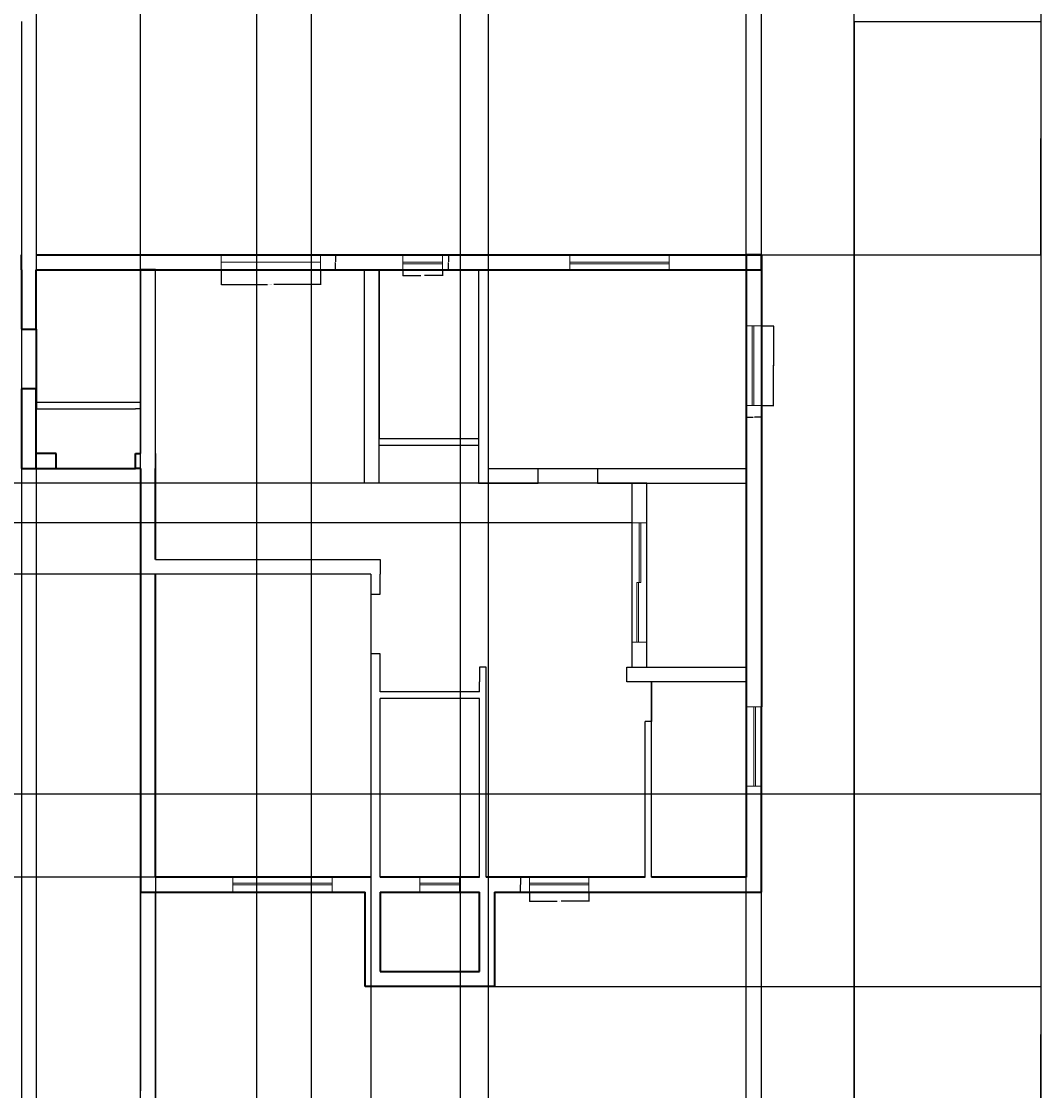
# Model space of a CAD drawing. Units: inches. Extents: x 2029 to 8798, y 1998 to 6373.
# Tile 9 of 11: x 3888 to 4504, y 5168 to 5814. Entities that reach past the tile are written whole.
import ezdxf

# ---------------------------------------------------------------- set-up
doc = ezdxf.new("R2010")
doc.units = ezdxf.units.IN
for name, color, linetype, lineweight in [('A-ANNO-DIMS', 2, 'Continuous', 18), ('A-GLAZ', 4, 'Continuous', 18), ('A-WALL-CIRC', 7, 'Continuous', 25), ('A-WALL-EXTR', 7, 'Continuous', 35), ('A-WALL-INTR', 7, 'Continuous', 25)]:
    doc.layers.add(name, color=color, linetype=linetype, lineweight=lineweight)
doc.styles.get("Standard").update_dxf_attribs({"font": 'arial.ttf'})
doc.dimstyles.get("Standard").update_dxf_attribs({"dimtxt": 0.18, "dimasz": 0.18, "dimexe": 0.18, "dimexo": 0.0625, "dimgap": 0.09, "dimtad": 0, "dimtih": 1, "dimtoh": 1, "dimdec": 4, "dimzin": 0, "dimdsep": 46, "dimtxsty": 'Standard', "dimcen": 0.09, "dimadec": 0, "dimazin": 0, "dimtfac": 1, "dimtdec": 4, "dimtofl": 0, "dimtmove": 0, "dimatfit": 3, "dimfxl": 1, "dimtolj": 1, "dimtzin": 0, "dimarcsym": 0})

# ---------------------------------------------------------------- blocks, each defined once
blk = doc.blocks.new('WIN-60')
for p, q in [((0, 0), (0, 9)), ((60, 9), (60, 0)), ((0, 4.5), (60, 4.5)), ((0, 3.5), (60, 3.5))]:
    blk.add_line(p, q)
blk = doc.blocks.new('WIN-36')
for p, q in [((0, 36), (9, 36)), ((3.5, 36), (3.5, 0)), ((4.5, 36), (4.5, 0)), ((9, 0), (0, 0))]:
    blk.add_line(p, q)
blk = doc.blocks.new('WIN-24')
for p, q in [((0, 0), (0, 9)), ((24, 9), (24, 0)), ((0, 4.5), (24, 4.5)), ((0, 3.5), (24, 3.5))]:
    blk.add_line(p, q)
blk = doc.blocks.new('WIN-48-DEEP-JAMB')
for p, q in [((9.38, 48), (0, 48)), ((0, 48), (0, 0)), ((3.69, 48), (3.69, 0)), ((4.69, 48), (4.69, 0)), ((0, 0), (9.38, 0))]:
    blk.add_line(p, q)
blk = doc.blocks.new('GLAZ-SLIDER-72-V')
for p, q in [((0, 72), (9, 72)), ((4.5, 72), (4.5, 36)), ((5.5, 72), (5.5, 36)), ((9, 72), (9, 0)), ((3, 36), (3, 0)), ((3, 36), (4, 36)), ((4, 36), (4, 0)), ((4.5, 36), (5.5, 36)), ((9, 0), (0, 0))]:
    blk.add_line(p, q)
blk = doc.blocks.new('WIN-60-SINGLE-LINE')
for p, q in [((0, 0), (0, 9)), ((0, 9), (60, 9)), ((60, 9), (60, 0)), ((0, 4.5), (60, 4.5))]:
    blk.add_line(p, q)
blk = doc.blocks.new('*D17')
at = {"layer": 'A-ANNO-DIMS', "color": 0, "lineweight": -2, "transparency": 16777216}
for p, q in [((4118.03, 5663.55), (4118.03, 5659.83)), ((4118.21, 5660.01), (4128.91, 5660.01)), ((4141.85, 5660.01), (4131.15, 5660.01)), ((4142.03, 5663.55), (4142.03, 5659.83))]:
    blk.add_line(p, q, dxfattribs=at)
at = {"layer": 'A-ANNO-DIMS', "color": 0, "transparency": 16777216}
for points in [[(4118.21, 5660.04), (4118.21, 5659.98), (4118.03, 5660.01)], [(4141.85, 5660.04), (4141.85, 5659.98), (4142.03, 5660.01)]]:
    blk.add_solid(points, dxfattribs=at)
at = {"layer": 'Defpoints', "color": 0, "transparency": 16777216}
for p in [(4118.03, 5663.61), (4142.03, 5663.61), (4142.03, 5660.01)]:
    blk.add_point(p, dxfattribs=at)
at = {"layer": 'A-ANNO-DIMS', "color": 0, "transparency": 16777216, "insert": (4130.03, 5660.01), "char_height": 0.18, "attachment_point": 5}
blk.add_mtext('\\A1;WINDOW 24 TYP.', dxfattribs=at)
blk = doc.blocks.new('*D18')
at = {"layer": 'A-ANNO-DIMS', "color": 0, "lineweight": -2, "transparency": 16777216}
for p, q in [((4142.1, 5672.61), (4145.81, 5672.61)), ((4145.63, 5672.43), (4145.63, 5668.29)), ((4145.63, 5663.79), (4145.63, 5667.93)), ((4142.1, 5663.61), (4145.81, 5663.61))]:
    blk.add_line(p, q, dxfattribs=at)
at = {"layer": 'A-ANNO-DIMS', "color": 0, "transparency": 16777216}
for points in [[(4145.6, 5672.43), (4145.66, 5672.43), (4145.63, 5672.61)], [(4145.6, 5663.79), (4145.66, 5663.79), (4145.63, 5663.61)]]:
    blk.add_solid(points, dxfattribs=at)
at = {"layer": 'Defpoints', "color": 0, "transparency": 16777216}
for p in [(4142.03, 5672.61), (4145.63, 5672.61), (4142.03, 5663.61)]:
    blk.add_point(p, dxfattribs=at)
at = {"layer": 'A-ANNO-DIMS', "color": 0, "transparency": 16777216, "insert": (4145.63, 5668.11), "char_height": 0.18, "attachment_point": 5}
blk.add_mtext('\\A1;9 TYP.', dxfattribs=at)
blk = doc.blocks.new('*D19')
at = {"layer": 'A-ANNO-DIMS', "color": 0, "lineweight": -2, "transparency": 16777216}
for p, q in [((4194.53, 5287.55), (4194.53, 5282.03)), ((4230.53, 5287.55), (4230.53, 5282.03)), ((4194.71, 5282.21), (4211.41, 5282.21)), ((4230.35, 5282.21), (4213.65, 5282.21))]:
    blk.add_line(p, q, dxfattribs=at)
at = {"layer": 'A-ANNO-DIMS', "color": 0, "transparency": 16777216}
for points in [[(4194.71, 5282.24), (4194.71, 5282.18), (4194.53, 5282.21)], [(4230.35, 5282.24), (4230.35, 5282.18), (4230.53, 5282.21)]]:
    blk.add_solid(points, dxfattribs=at)
at = {"layer": 'Defpoints', "color": 0, "transparency": 16777216}
for p in [(4194.53, 5287.61), (4230.53, 5287.61), (4230.53, 5282.21)]:
    blk.add_point(p, dxfattribs=at)
at = {"layer": 'A-ANNO-DIMS', "color": 0, "transparency": 16777216, "insert": (4212.53, 5282.21), "char_height": 0.18, "attachment_point": 5}
blk.add_mtext('\\A1;WINDOW 36 TYP.', dxfattribs=at)
blk = doc.blocks.new('*D20')
at = {"layer": 'A-ANNO-DIMS', "color": 0, "lineweight": -2, "transparency": 16777216}
for p, q in [((4194.47, 5296.61), (4188.95, 5296.61)), ((4189.13, 5296.43), (4189.13, 5292.29)), ((4189.13, 5287.79), (4189.13, 5291.93)), ((4194.47, 5287.61), (4188.95, 5287.61))]:
    blk.add_line(p, q, dxfattribs=at)
at = {"layer": 'A-ANNO-DIMS', "color": 0, "transparency": 16777216}
for points in [[(4189.1, 5296.43), (4189.16, 5296.43), (4189.13, 5296.61)], [(4189.1, 5287.79), (4189.16, 5287.79), (4189.13, 5287.61)]]:
    blk.add_solid(points, dxfattribs=at)
at = {"layer": 'Defpoints', "color": 0, "transparency": 16777216}
for p in [(4194.53, 5296.61), (4189.13, 5287.61), (4194.53, 5287.61)]:
    blk.add_point(p, dxfattribs=at)
at = {"layer": 'A-ANNO-DIMS', "color": 0, "transparency": 16777216, "insert": (4189.13, 5292.11), "char_height": 0.18, "attachment_point": 5}
blk.add_mtext('\\A1;9 TYP.', dxfattribs=at)
blk = doc.blocks.new('*D23')
at = {"layer": 'A-ANNO-DIMS', "color": 0, "lineweight": -2, "transparency": 16777216}
for p, q in [((4334.83, 5629.66), (4342.15, 5629.66)), ((4341.97, 5629.48), (4341.97, 5605.84)), ((4341.97, 5581.84), (4341.97, 5605.48)), ((4334.83, 5581.66), (4342.15, 5581.66))]:
    blk.add_line(p, q, dxfattribs=at)
at = {"layer": 'A-ANNO-DIMS', "color": 0, "transparency": 16777216}
for points in [[(4341.94, 5629.48), (4342, 5629.48), (4341.97, 5629.66)], [(4341.94, 5581.84), (4342, 5581.84), (4341.97, 5581.66)]]:
    blk.add_solid(points, dxfattribs=at)
at = {"layer": 'Defpoints', "color": 0, "transparency": 16777216}
for p in [(4334.77, 5629.66), (4341.97, 5629.66), (4334.77, 5581.66)]:
    blk.add_point(p, dxfattribs=at)
at = {"layer": 'A-ANNO-DIMS', "color": 0, "transparency": 16777216, "insert": (4341.97, 5605.66), "char_height": 0.18, "attachment_point": 5}
blk.add_mtext('\\A1;DEEP JAMB 48 TYP.', dxfattribs=at)
blk = doc.blocks.new('*D24')
at = {"layer": 'A-ANNO-DIMS', "color": 0, "lineweight": -2, "transparency": 16777216}
for p, q in [((4325.39, 5581.6), (4325.39, 5574.28)), ((4334.77, 5581.6), (4334.77, 5574.28)), ((4325.57, 5574.46), (4329.62, 5574.46)), ((4334.59, 5574.46), (4330.53, 5574.46))]:
    blk.add_line(p, q, dxfattribs=at)
at = {"layer": 'A-ANNO-DIMS', "color": 0, "transparency": 16777216}
for points in [[(4325.57, 5574.49), (4325.57, 5574.43), (4325.39, 5574.46)], [(4334.59, 5574.49), (4334.59, 5574.43), (4334.77, 5574.46)]]:
    blk.add_solid(points, dxfattribs=at)
at = {"layer": 'Defpoints', "color": 0, "transparency": 16777216}
for p in [(4325.39, 5581.66), (4334.77, 5581.66), (4334.77, 5574.46)]:
    blk.add_point(p, dxfattribs=at)
at = {"layer": 'A-ANNO-DIMS', "color": 0, "transparency": 16777216, "insert": (4330.08, 5574.46), "char_height": 0.18, "attachment_point": 5}
blk.add_mtext('\\A1;9 TYP.', dxfattribs=at)
blk = doc.blocks.new('*D33')
at = {"layer": 'A-ANNO-DIMS', "color": 0, "lineweight": -2, "transparency": 16777216}
for p, q in [((4008.38, 5663.55), (4008.38, 5654.43)), ((4068.38, 5663.55), (4068.38, 5654.43)), ((4008.56, 5654.61), (4036.45, 5654.61)), ((4068.2, 5654.61), (4040.32, 5654.61))]:
    blk.add_line(p, q, dxfattribs=at)
at = {"layer": 'A-ANNO-DIMS', "color": 0, "transparency": 16777216}
for points in [[(4008.56, 5654.64), (4008.56, 5654.58), (4008.38, 5654.61)], [(4068.2, 5654.64), (4068.2, 5654.58), (4068.38, 5654.61)]]:
    blk.add_solid(points, dxfattribs=at)
at = {"layer": 'Defpoints', "color": 0, "transparency": 16777216}
for p in [(4008.38, 5663.61), (4068.38, 5663.61), (4068.38, 5654.61)]:
    blk.add_point(p, dxfattribs=at)
at = {"layer": 'A-ANNO-DIMS', "color": 0, "transparency": 16777216, "insert": (4038.38, 5654.61), "char_height": 0.18, "attachment_point": 5}
blk.add_mtext('\\A1;SINGLE-LINE WINDOW 60 TYP.', dxfattribs=at)
blk = doc.blocks.new('*D34')
at = {"layer": 'A-ANNO-DIMS', "color": 0, "lineweight": -2, "transparency": 16777216}
for p, q in [((4068.45, 5672.61), (4077.56, 5672.61)), ((4077.38, 5672.43), (4077.38, 5668.29)), ((4077.38, 5663.79), (4077.38, 5667.93)), ((4068.45, 5663.61), (4077.56, 5663.61))]:
    blk.add_line(p, q, dxfattribs=at)
at = {"layer": 'A-ANNO-DIMS', "color": 0, "transparency": 16777216}
for points in [[(4077.35, 5672.43), (4077.41, 5672.43), (4077.38, 5672.61)], [(4077.35, 5663.79), (4077.41, 5663.79), (4077.38, 5663.61)]]:
    blk.add_solid(points, dxfattribs=at)
at = {"layer": 'Defpoints', "color": 0, "transparency": 16777216}
for p in [(4068.38, 5672.61), (4077.38, 5672.61), (4068.38, 5663.61)]:
    blk.add_point(p, dxfattribs=at)
at = {"layer": 'A-ANNO-DIMS', "color": 0, "transparency": 16777216, "insert": (4077.38, 5668.11), "char_height": 0.18, "attachment_point": 5}
blk.add_mtext('\\A1;9 TYP.', dxfattribs=at)
blk = doc.blocks.new('*D60')
at = {"layer": 'A-ANNO-DIMS', "color": 0, "lineweight": -2, "transparency": 16777216}
for p, q in [((3414.59, 5346.99), (4503.7, 5346.99)), ((4503.52, 5346.81), (4503.52, 5150.67)), ((4503.52, 4954.17), (4503.52, 5150.31)), ((3414.59, 4953.99), (4503.7, 4953.99))]:
    blk.add_line(p, q, dxfattribs=at)
at = {"layer": 'A-ANNO-DIMS', "color": 0, "transparency": 16777216}
for points in [[(4503.49, 5346.81), (4503.55, 5346.81), (4503.52, 5346.99)], [(4503.49, 4954.17), (4503.55, 4954.17), (4503.52, 4953.99)]]:
    blk.add_solid(points, dxfattribs=at)
at = {"layer": 'Defpoints', "color": 0, "transparency": 16777216}
for p in [(3414.53, 5346.99), (4503.52, 5346.99), (3414.53, 4953.99)]:
    blk.add_point(p, dxfattribs=at)
at = {"layer": 'A-ANNO-DIMS', "color": 0, "transparency": 16777216, "insert": (4503.52, 5150.49), "char_height": 0.18, "attachment_point": 5}
blk.add_mtext('\\A1;393', dxfattribs=at)
blk = doc.blocks.new('*D73')
at = {"layer": 'A-ANNO-DIMS', "color": 0, "lineweight": -2, "transparency": 16777216}
for p, q in [((4173.45, 5230.61), (4503.7, 5230.61)), ((4503.52, 5230.43), (4503.52, 5176.04)), ((4503.52, 5121.27), (4503.52, 5175.67)), ((4334.83, 5121.09), (4503.7, 5121.09))]:
    blk.add_line(p, q, dxfattribs=at)
at = {"layer": 'A-ANNO-DIMS', "color": 0, "transparency": 16777216}
for points in [[(4503.49, 5230.43), (4503.55, 5230.43), (4503.52, 5230.61)], [(4503.49, 5121.27), (4503.55, 5121.27), (4503.52, 5121.09)]]:
    blk.add_solid(points, dxfattribs=at)
at = {"layer": 'Defpoints', "color": 0, "transparency": 16777216}
for p in [(4173.39, 5230.61), (4503.52, 5230.61), (4334.77, 5121.09)]:
    blk.add_point(p, dxfattribs=at)
at = {"layer": 'A-ANNO-DIMS', "color": 0, "transparency": 16777216, "insert": (4503.52, 5175.85), "char_height": 0.18, "attachment_point": 5}
blk.add_mtext('\\A1;109.52', dxfattribs=at)
blk = doc.blocks.new('*D74')
at = {"layer": 'A-ANNO-DIMS', "color": 0, "lineweight": -2, "transparency": 16777216}
for p, q in [((4390.83, 5813.61), (4503.7, 5813.61)), ((4503.52, 5813.43), (4503.52, 5743.29)), ((4503.52, 5672.79), (4503.52, 5742.93)), ((4334.83, 5672.61), (4503.7, 5672.61))]:
    blk.add_line(p, q, dxfattribs=at)
at = {"layer": 'A-ANNO-DIMS', "color": 0, "transparency": 16777216}
for points in [[(4503.49, 5813.43), (4503.55, 5813.43), (4503.52, 5813.61)], [(4503.49, 5672.79), (4503.55, 5672.79), (4503.52, 5672.61)]]:
    blk.add_solid(points, dxfattribs=at)
at = {"layer": 'Defpoints', "color": 0, "transparency": 16777216}
for p in [(4390.77, 5813.61), (4503.52, 5813.61), (4334.77, 5672.61)]:
    blk.add_point(p, dxfattribs=at)
at = {"layer": 'A-ANNO-DIMS', "color": 0, "transparency": 16777216, "insert": (4503.52, 5743.11), "char_height": 0.18, "attachment_point": 5}
blk.add_mtext('\\A1;141', dxfattribs=at)
blk = doc.blocks.new('*D76')
at = {"layer": 'A-ANNO-DIMS', "color": 0, "lineweight": -2, "transparency": 16777216}
for p, q in [((3887.77, 5813.55), (3887.77, 4031.06)), ((4390.77, 5813.55), (4390.77, 4031.06)), ((3887.95, 4031.24), (4138.98, 4031.24)), ((4390.59, 4031.24), (4139.55, 4031.24))]:
    blk.add_line(p, q, dxfattribs=at)
at = {"layer": 'A-ANNO-DIMS', "color": 0, "transparency": 16777216}
for points in [[(3887.95, 4031.27), (3887.95, 4031.21), (3887.77, 4031.24)], [(4390.59, 4031.27), (4390.59, 4031.21), (4390.77, 4031.24)]]:
    blk.add_solid(points, dxfattribs=at)
at = {"layer": 'Defpoints', "color": 0, "transparency": 16777216}
for p in [(3887.77, 5813.61), (4390.77, 5813.61), (4390.77, 4031.24)]:
    blk.add_point(p, dxfattribs=at)
at = {"layer": 'A-ANNO-DIMS', "color": 0, "transparency": 16777216, "insert": (4139.27, 4031.24), "char_height": 0.18, "attachment_point": 5}
blk.add_mtext('\\A1;503', dxfattribs=at)
blk = doc.blocks.new('*D77')
at = {"layer": 'A-ANNO-DIMS', "color": 0, "lineweight": -2, "transparency": 16777216}
for p, q in [((3959.77, 5121.16), (3959.77, 6372.54)), ((3959.95, 6372.36), (4146.98, 6372.36)), ((4334.59, 6372.36), (4147.56, 6372.36)), ((4334.77, 5121.16), (4334.77, 6372.54))]:
    blk.add_line(p, q, dxfattribs=at)
at = {"layer": 'A-ANNO-DIMS', "color": 0, "transparency": 16777216}
for points in [[(3959.95, 6372.39), (3959.95, 6372.33), (3959.77, 6372.36)], [(4334.59, 6372.39), (4334.59, 6372.33), (4334.77, 6372.36)]]:
    blk.add_solid(points, dxfattribs=at)
at = {"layer": 'Defpoints', "color": 0, "transparency": 16777216}
for p in [(4334.77, 6372.36), (3959.77, 5121.09), (4334.77, 5121.09)]:
    blk.add_point(p, dxfattribs=at)
at = {"layer": 'A-ANNO-DIMS', "color": 0, "transparency": 16777216, "insert": (4147.27, 6372.36), "char_height": 0.18, "attachment_point": 5}
blk.add_mtext('\\A1;375', dxfattribs=at)
blk = doc.blocks.new('*D78')
at = {"layer": 'A-ANNO-DIMS', "color": 0, "lineweight": -2, "transparency": 16777216}
for p, q in [((3896.77, 6211.55), (3896.77, 4031.06)), ((4029.77, 6211.55), (4029.77, 4031.06)), ((3896.95, 4031.24), (3962.99, 4031.24)), ((4029.59, 4031.24), (3963.55, 4031.24))]:
    blk.add_line(p, q, dxfattribs=at)
at = {"layer": 'A-ANNO-DIMS', "color": 0, "transparency": 16777216}
for points in [[(3896.95, 4031.27), (3896.95, 4031.21), (3896.77, 4031.24)], [(4029.59, 4031.27), (4029.59, 4031.21), (4029.77, 4031.24)]]:
    blk.add_solid(points, dxfattribs=at)
at = {"layer": 'Defpoints', "color": 0, "transparency": 16777216}
for p in [(3896.77, 6211.61), (4029.77, 6211.61), (4029.77, 4031.24)]:
    blk.add_point(p, dxfattribs=at)
at = {"layer": 'A-ANNO-DIMS', "color": 0, "transparency": 16777216, "insert": (3963.27, 4031.24), "char_height": 0.18, "attachment_point": 5}
blk.add_mtext('\\A1;133', dxfattribs=at)
blk = doc.blocks.new('*D83')
at = {"layer": 'A-ANNO-DIMS', "color": 0, "lineweight": -2, "transparency": 16777216}
for p, q in [((4062.77, 6151.55), (4062.77, 4031.06)), ((4152.77, 6151.55), (4152.77, 4031.06)), ((4062.95, 4031.24), (4107.55, 4031.24)), ((4152.59, 4031.24), (4107.98, 4031.24))]:
    blk.add_line(p, q, dxfattribs=at)
at = {"layer": 'A-ANNO-DIMS', "color": 0, "transparency": 16777216}
for points in [[(4062.95, 4031.27), (4062.95, 4031.21), (4062.77, 4031.24)], [(4152.59, 4031.27), (4152.59, 4031.21), (4152.77, 4031.24)]]:
    blk.add_solid(points, dxfattribs=at)
at = {"layer": 'Defpoints', "color": 0, "transparency": 16777216}
for p in [(4062.77, 6151.61), (4152.77, 6151.61), (4152.77, 4031.24)]:
    blk.add_point(p, dxfattribs=at)
at = {"layer": 'A-ANNO-DIMS', "color": 0, "transparency": 16777216, "insert": (4107.77, 4031.24), "char_height": 0.18, "attachment_point": 5}
blk.add_mtext('\\A1;90', dxfattribs=at)
blk = doc.blocks.new('*D88')
at = {"layer": 'A-ANNO-DIMS', "color": 0, "lineweight": -2, "transparency": 16777216}
for p, q in [((2142.54, 4445.05), (2142.54, 6372.54)), ((2142.72, 6372.36), (3266.19, 6372.36)), ((4390.59, 6372.36), (3267.12, 6372.36)), ((4390.77, 4574.05), (4390.77, 6372.54))]:
    blk.add_line(p, q, dxfattribs=at)
at = {"layer": 'A-ANNO-DIMS', "color": 0, "transparency": 16777216}
for points in [[(2142.72, 6372.39), (2142.72, 6372.33), (2142.54, 6372.36)], [(4390.59, 6372.39), (4390.59, 6372.33), (4390.77, 6372.36)]]:
    blk.add_solid(points, dxfattribs=at)
at = {"layer": 'Defpoints', "color": 0, "transparency": 16777216}
for p in [(4390.77, 6372.36), (4390.77, 4573.99), (2142.54, 4444.99)]:
    blk.add_point(p, dxfattribs=at)
at = {"layer": 'A-ANNO-DIMS', "color": 0, "transparency": 16777216, "insert": (3266.65, 6372.36), "char_height": 0.18, "attachment_point": 5}
blk.add_mtext('\\A1;2248.2', dxfattribs=at)
blk = doc.blocks.new('*D89')
at = {"layer": 'A-ANNO-DIMS', "color": 0, "lineweight": -2, "transparency": 16777216}
for p, q in [((4249.83, 6259.61), (4503.7, 6259.61)), ((4503.52, 6259.43), (4503.52, 5201.98)), ((4503.52, 4144.17), (4503.52, 5201.62)), ((4105.83, 4143.99), (4503.7, 4143.99))]:
    blk.add_line(p, q, dxfattribs=at)
at = {"layer": 'A-ANNO-DIMS', "color": 0, "transparency": 16777216}
for points in [[(4503.49, 6259.43), (4503.55, 6259.43), (4503.52, 6259.61)], [(4503.49, 4144.17), (4503.55, 4144.17), (4503.52, 4143.99)]]:
    blk.add_solid(points, dxfattribs=at)
at = {"layer": 'Defpoints', "color": 0, "transparency": 16777216}
for p in [(4249.77, 6259.61), (4503.52, 6259.61), (4105.77, 4143.99)]:
    blk.add_point(p, dxfattribs=at)
at = {"layer": 'A-ANNO-DIMS', "color": 0, "transparency": 16777216, "insert": (4503.52, 5201.8), "char_height": 0.18, "attachment_point": 5}
blk.add_mtext('\\A1;2115.6', dxfattribs=at)
blk = doc.blocks.new('*D105')
at = {"layer": 'A-ANNO-DIMS', "color": 0, "lineweight": -2, "transparency": 16777216}
for p, q in [((3968.7, 5479.61), (2029.61, 5479.61)), ((2029.79, 5479.43), (2029.79, 5388.29)), ((2029.79, 5296.79), (2029.79, 5387.93)), ((3968.7, 5296.61), (2029.61, 5296.61))]:
    blk.add_line(p, q, dxfattribs=at)
at = {"layer": 'A-ANNO-DIMS', "color": 0, "transparency": 16777216}
for points in [[(2029.76, 5479.43), (2029.82, 5479.43), (2029.79, 5479.61)], [(2029.76, 5296.79), (2029.82, 5296.79), (2029.79, 5296.61)]]:
    blk.add_solid(points, dxfattribs=at)
at = {"layer": 'Defpoints', "color": 0, "transparency": 16777216}
for p in [(2029.79, 5479.61), (3968.77, 5479.61), (3968.77, 5296.61)]:
    blk.add_point(p, dxfattribs=at)
at = {"layer": 'A-ANNO-DIMS', "color": 0, "transparency": 16777216, "insert": (2029.79, 5388.11), "char_height": 0.18, "attachment_point": 5}
blk.add_mtext('\\A1;183', dxfattribs=at)
blk = doc.blocks.new('*D107')
at = {"layer": 'A-ANNO-DIMS', "color": 0, "lineweight": -2, "transparency": 16777216}
for p, q in [((3968.77, 5479.55), (3968.77, 4031.06)), ((4098.77, 5479.55), (4098.77, 4031.06)), ((3968.95, 4031.24), (4033.49, 4031.24)), ((4098.59, 4031.24), (4034.05, 4031.24))]:
    blk.add_line(p, q, dxfattribs=at)
at = {"layer": 'A-ANNO-DIMS', "color": 0, "transparency": 16777216}
for points in [[(3968.95, 4031.27), (3968.95, 4031.21), (3968.77, 4031.24)], [(4098.59, 4031.27), (4098.59, 4031.21), (4098.77, 4031.24)]]:
    blk.add_solid(points, dxfattribs=at)
at = {"layer": 'Defpoints', "color": 0, "transparency": 16777216}
for p in [(3968.77, 5479.61), (4098.77, 5479.61), (4098.77, 4031.24)]:
    blk.add_point(p, dxfattribs=at)
at = {"layer": 'A-ANNO-DIMS', "color": 0, "transparency": 16777216, "insert": (4033.77, 4031.24), "char_height": 0.18, "attachment_point": 5}
blk.add_mtext('\\A1;130', dxfattribs=at)
blk = doc.blocks.new('*D108')
at = {"layer": 'A-ANNO-DIMS', "color": 0, "lineweight": -2, "transparency": 16777216}
for p, q in [((4256.32, 5534.61), (2029.61, 5534.61)), ((2029.79, 5534.43), (2029.79, 5522.79)), ((2029.79, 5510.79), (2029.79, 5522.43)), ((4256.32, 5510.61), (2029.61, 5510.61))]:
    blk.add_line(p, q, dxfattribs=at)
at = {"layer": 'A-ANNO-DIMS', "color": 0, "transparency": 16777216}
for points in [[(2029.76, 5534.43), (2029.82, 5534.43), (2029.79, 5534.61)], [(2029.76, 5510.79), (2029.82, 5510.79), (2029.79, 5510.61)]]:
    blk.add_solid(points, dxfattribs=at)
at = {"layer": 'Defpoints', "color": 0, "transparency": 16777216}
for p in [(4256.39, 5534.61), (2029.79, 5510.61), (4256.39, 5510.61)]:
    blk.add_point(p, dxfattribs=at)
at = {"layer": 'A-ANNO-DIMS', "color": 0, "transparency": 16777216, "insert": (2029.79, 5522.61), "char_height": 0.18, "attachment_point": 5}
blk.add_mtext('\\A1;24', dxfattribs=at)
blk = doc.blocks.new('*D109')
at = {"layer": 'A-ANNO-DIMS', "color": 0, "lineweight": -2, "transparency": 16777216}
for p, q in [((4169.77, 4992.16), (4169.77, 6372.54)), ((4169.95, 6372.36), (4247.12, 6372.36)), ((4325.21, 6372.36), (4248.03, 6372.36)), ((4325.39, 4992.16), (4325.39, 6372.54))]:
    blk.add_line(p, q, dxfattribs=at)
at = {"layer": 'A-ANNO-DIMS', "color": 0, "transparency": 16777216}
for points in [[(4169.95, 6372.39), (4169.95, 6372.33), (4169.77, 6372.36)], [(4325.21, 6372.39), (4325.21, 6372.33), (4325.39, 6372.36)]]:
    blk.add_solid(points, dxfattribs=at)
at = {"layer": 'Defpoints', "color": 0, "transparency": 16777216}
for p in [(4325.39, 6372.36), (4169.77, 4992.09), (4325.39, 4992.09)]:
    blk.add_point(p, dxfattribs=at)
at = {"layer": 'A-ANNO-DIMS', "color": 0, "transparency": 16777216, "insert": (4247.58, 6372.36), "char_height": 0.18, "attachment_point": 5}
blk.add_mtext('\\A1;155.62', dxfattribs=at)

msp = doc.modelspace()

# ---------------------------------------------------------------- linework, layer by layer
at = {"layer": 'A-GLAZ'}
for p, q in [((4118.0329, 5672.6123), (4142.0329, 5672.6123)), ((4218.9796, 5672.6123), (4278.9796, 5672.6123)), ((4075.4621, 5287.6123), (4015.4621, 5287.6123)), ((4152.3869, 5287.6123), (4128.3869, 5287.6123)), ((4230.5315, 5287.6123), (4194.5315, 5287.6123))]:
    msp.add_line(p, q, dxfattribs=at)
at = {"layer": 'A-WALL-CIRC'}
for p, q in [((3896.7657, 5822.6123), (3896.7657, 5672.6123)), ((3887.7657, 5813.6123), (3887.7657, 5663.6123)), ((3959.7657, 5287.6123), (3959.7657, 5167.6123)), ((3968.7657, 5107.6123), (3968.7657, 5287.6123))]:
    msp.add_line(p, q, dxfattribs=at)
at = {"layer": 'A-WALL-EXTR'}
for p, q in [((3887.7657, 5663.6123), (3887.7657, 5672.6123)), ((3896.7657, 5672.6123), (4334.3869, 5672.6123)), ((4334.3869, 5672.6123), (4325.3869, 5672.6123)), ((4325.3869, 5672.6123), (4325.3869, 5399.6123)), ((4334.7657, 5672.6123), (4332.4986, 5672.6123)), ((4334.7657, 5663.6123), (4334.7657, 5672.6123)), ((4334.7657, 5672.6123), (4334.7657, 5399.6123)), ((3887.7657, 5663.6123), (3887.7657, 5627.6123)), ((3896.7657, 5627.6123), (3896.7657, 5663.6123)), ((3896.7657, 5663.6123), (4094.7657, 5663.6123)), ((3968.7657, 5663.6123), (3959.7657, 5663.6123)), ((3968.7657, 5663.6123), (4094.7657, 5663.6123)), ((3968.7657, 5663.6123), (4008.3833, 5663.6123)), ((3991.2657, 5663.6123), (4097.1962, 5663.6123)), ((4094.7657, 5663.6123), (4334.7657, 5663.6123)), ((4103.7657, 5663.6123), (4163.7657, 5663.6123)), ((4103.7657, 5663.6123), (4118.0329, 5663.6123)), ((4169.7657, 5663.6123), (4218.9796, 5663.6123)), ((4334.7657, 5663.6123), (4334.7657, 5629.6619)), ((3887.7657, 5627.6123), (3896.7657, 5627.6123)), ((3896.7657, 5627.6123), (3896.7657, 5591.6123)), ((3896.7657, 5591.6123), (3887.7657, 5591.6123)), ((3887.7657, 5591.6123), (3887.7657, 5543.6123)), ((3896.7657, 5543.6123), (3896.7657, 5591.6123)), ((3896.7657, 5591.6123), (3896.7657, 5579.6123)), ((3908.7657, 5552.6123), (3896.7657, 5552.6123)), ((3908.7657, 5543.6123), (3908.7657, 5552.6123)), ((3956.7657, 5543.6123), (3956.7657, 5552.6123)), ((3956.7657, 5552.6123), (3959.7657, 5552.6123)), ((3887.7657, 5543.6123), (3896.7657, 5543.6123)), ((3896.7657, 5543.6123), (3908.7657, 5543.6123)), ((3908.7657, 5543.6123), (3956.7657, 5543.6123)), ((3959.7657, 5543.6123), (3956.7657, 5543.6123)), ((3959.7657, 5543.6123), (3956.7657, 5543.6123)), ((3959.7657, 5543.6123), (3959.7657, 5287.6123)), ((3968.7657, 5488.6123), (3968.7657, 5543.6123)), ((4325.3869, 5534.6123), (4325.3869, 5414.6123)), ((3968.7657, 5488.6123), (3968.7657, 5488.6123)), ((3968.7657, 5296.6123), (3968.7657, 5479.6123)), ((3968.7657, 5296.6123), (3968.7657, 5479.6123)), ((4325.3869, 5414.6123), (4325.3869, 5296.6123)), ((4334.7657, 5296.6123), (4334.7657, 5399.6123)), ((4098.7657, 5296.6123), (3968.7657, 5296.6123)), ((4098.7657, 5296.6123), (4075.4621, 5296.6123)), ((4164.3869, 5296.6123), (4104.3869, 5296.6123)), ((4160.3869, 5296.6123), (4104.3869, 5296.6123)), ((4164.3869, 5296.6123), (4104.3869, 5296.6123)), ((4164.3869, 5296.6123), (4104.3869, 5296.6123)), ((4164.3869, 5296.6123), (4152.3869, 5296.6123)), ((4262.3869, 5296.6123), (4168.3869, 5296.6123)), ((4262.3869, 5296.6123), (4168.3869, 5296.6123)), ((4262.3869, 5296.6123), (4230.5315, 5296.6123)), ((4264.3869, 5296.6123), (4262.3869, 5296.6123)), ((4325.3869, 5296.6123), (4268.3869, 5296.6123)), ((4325.3869, 5296.6123), (4268.3869, 5296.6123)), ((4334.7657, 5287.6123), (4334.7657, 5296.6123)), ((3959.7657, 5287.6123), (4095.3869, 5287.6123)), ((4095.3869, 5230.6123), (4095.3869, 5287.6123)), ((4104.3869, 5287.6123), (4104.3869, 5239.6123)), ((4104.3869, 5287.6123), (4164.3869, 5287.6123)), ((4164.3869, 5239.6123), (4164.3869, 5287.6123)), ((4173.3869, 5287.6123), (4173.3869, 5230.6123)), ((4173.3869, 5287.6123), (4334.7657, 5287.6123)), ((4104.3869, 5239.6123), (4128.3869, 5239.6123)), ((4128.3869, 5239.6123), (4164.3869, 5239.6123)), ((4104.3869, 5230.6123), (4095.3869, 5230.6123)), ((4128.3869, 5230.6123), (4104.3869, 5230.6123)), ((4173.3869, 5230.6123), (4128.3869, 5230.6123))]:
    msp.add_line(p, q, dxfattribs=at)
at = {"layer": 'A-WALL-INTR'}
for p, q in [((3959.7657, 5663.6123), (3959.7657, 5552.6123)), ((3968.7657, 5543.6123), (3968.7657, 5663.6123)), ((4094.7657, 5663.6123), (4094.7657, 5534.6123)), ((4103.7657, 5534.6123), (4103.7657, 5663.6123)), ((4103.7657, 5663.6123), (4103.7657, 5561.6123)), ((4163.7657, 5663.6123), (4163.7657, 5543.6123)), ((4169.7657, 5543.6123), (4169.7657, 5663.6123)), ((3896.7657, 5583.6123), (3956.7657, 5583.6123)), ((3956.7657, 5583.6123), (3959.7657, 5583.6123)), ((3959.7657, 5583.6123), (3959.7657, 5579.5975)), ((3896.7657, 5579.6123), (3956.7657, 5579.6123)), ((3959.7657, 5579.5975), (3956.7657, 5579.6123)), ((4103.7657, 5561.6123), (4163.7657, 5561.6123)), ((4103.7657, 5557.6123), (4163.7657, 5557.6123)), ((3968.7657, 5552.6123), (3968.7657, 5543.6123)), ((4163.7657, 5543.6123), (4163.7657, 5534.6123)), ((4169.7657, 5543.6123), (4325.3869, 5543.6123)), ((4199.7657, 5534.6123), (4199.7657, 5543.6123)), ((4199.7657, 5543.6123), (4235.7657, 5543.6123)), ((4235.7657, 5543.6123), (4235.7657, 5534.6123)), ((4103.7657, 5534.6123), (4094.7657, 5534.6123)), ((4163.7657, 5534.6123), (4103.7657, 5534.6123)), ((4163.7657, 5534.6123), (4169.7657, 5534.6123)), ((4163.7657, 5534.6123), (4199.7657, 5534.6123)), ((4169.7657, 5534.6123), (4199.7657, 5534.6123)), ((4235.7657, 5534.6123), (4325.3869, 5534.6123)), ((4265.3869, 5534.6123), (4256.3869, 5534.6123)), ((4256.3869, 5534.6123), (4256.3869, 5423.6123)), ((4256.3869, 5534.6123), (4256.3869, 5510.6123)), ((4265.3869, 5423.6123), (4265.3869, 5534.6123)), ((3968.7657, 5488.6123), (4104.3869, 5488.6123)), ((4104.3869, 5488.6123), (4104.3869, 5479.6123)), ((4098.7657, 5479.6123), (3968.7657, 5479.6123)), ((4098.7657, 5479.6123), (4098.7657, 5296.6123)), ((4098.7657, 5479.6123), (4098.7657, 5467.6123)), ((4104.3869, 5467.6123), (4104.3869, 5479.6123)), ((4098.7657, 5467.6123), (4104.3869, 5467.6123)), ((4104.3869, 5431.6123), (4098.7657, 5431.6123)), ((4104.3869, 5408.6123), (4104.3869, 5431.6123)), ((4168.3869, 5423.6123), (4164.3869, 5423.6123)), ((4164.3869, 5423.6123), (4164.3869, 5414.6123)), ((4168.3869, 5414.6123), (4168.3869, 5423.6123)), ((4253.3869, 5414.6123), (4253.3869, 5423.6123)), ((4253.3869, 5423.6123), (4265.3869, 5423.6123)), ((4265.3869, 5423.6123), (4325.3869, 5423.6123)), ((4164.3869, 5408.6123), (4164.3869, 5414.6123)), ((4168.3869, 5296.6123), (4168.3869, 5414.6123)), ((4325.3869, 5414.6123), (4253.3869, 5414.6123)), ((4268.3869, 5414.6123), (4264.3869, 5414.6123)), ((4268.3869, 5296.6123), (4268.3869, 5414.6123)), ((4268.3869, 5414.6123), (4268.3869, 5390.6123)), ((4164.3869, 5408.6123), (4104.3869, 5408.6123)), ((4104.3869, 5296.6123), (4104.3869, 5404.6123)), ((4164.3869, 5404.6123), (4104.3869, 5404.6123)), ((4164.3869, 5296.6123), (4164.3869, 5404.6123)), ((4164.3869, 5296.6123), (4164.3869, 5404.6123)), ((4264.3869, 5296.6123), (4264.3869, 5390.6123)), ((4268.3869, 5390.6123), (4264.3869, 5390.6123))]:
    msp.add_line(p, q, dxfattribs=at)

# ---------------------------------------------------------------- block references
at = {"layer": 'A-GLAZ'}
for name, p in [('WIN-60-SINGLE-LINE', (4008.3833, 5663.6123)), ('WIN-24', (4118.0329, 5663.6123)), ('WIN-60', (4218.9796, 5663.6123)), ('WIN-48-DEEP-JAMB', (4325.3869, 5581.6619)), ('GLAZ-SLIDER-72-V', (4256.3869, 5438.6123))]:
    msp.add_blockref(name, p, dxfattribs=at)
at = {"layer": 'A-GLAZ', "extrusion": (0, 0, -1), "zscale": -1}
msp.add_blockref('WIN-48-DEEP-JAMB', (-4334.7657, 5351.6123), dxfattribs=at)
at = {"layer": 'A-GLAZ', "extrusion": (0, 0, -1), "zscale": -1, "rotation": 180}
for name, p in [('WIN-60', (-4015.4621, 5296.6123)), ('WIN-24', (-4128.3869, 5296.6123))]:
    msp.add_blockref(name, p, dxfattribs=at)
at = {"layer": 'A-GLAZ', "rotation": 270}
msp.add_blockref('WIN-36', (4194.5315, 5296.6123), dxfattribs=at)

# ---------------------------------------------------------------- dimensions: what is measured, and where the dimension line sits
at = {"layer": 'A-ANNO-DIMS'}
for base, p1, p2, override, picture, middle in [((4390.7657, 6372.3623), (2142.5398, 4444.9886), (4390.7657, 4573.9886), {"dimdec": 1, "dimlfac": 1, "dimrnd": 0, "dimzin": 0, "dimdsep": 46, "dimlunit": 2}, '*D88', (3266.6528, 6372.3623)), ((4334.7657, 6372.3623), (3959.7657, 5121.0948), (4334.7657, 5121.0948), {"dimdec": 0, "dimlfac": 1, "dimrnd": 0, "dimzin": 0, "dimdsep": 46, "dimlunit": 2}, '*D77', (4147.2657, 6372.3623)), ((4325.3869, 6372.3623), (4169.7657, 4992.0948), (4325.3869, 4992.0948), {"dimdec": 2, "dimlfac": 1, "dimrnd": 0, "dimzin": 0, "dimdsep": 46, "dimlunit": 2}, '*D109', (4247.5763, 6372.3623)), ((4029.7657, 4031.2386), (3896.7657, 6211.6123), (4029.7657, 6211.6123), {"dimdec": 0, "dimlfac": 1, "dimrnd": 0, "dimzin": 0, "dimdsep": 46, "dimlunit": 2}, '*D78', (3963.2657, 4031.2386)), ((4152.7657, 4031.2386), (4062.7657, 6151.6123), (4152.7657, 6151.6123), {"dimdec": 0, "dimlfac": 1, "dimrnd": 0, "dimzin": 0, "dimdsep": 46, "dimlunit": 2}, '*D83', (4107.7657, 4031.2386)), ((4390.7657, 4031.2386), (3887.7657, 5813.6123), (4390.7657, 5813.6123), {"dimdec": 0, "dimlfac": 1, "dimrnd": 0, "dimzin": 0, "dimdsep": 46, "dimlunit": 2}, '*D76', (4139.2657, 4031.2386)), ((4098.7657, 4031.2386), (3968.7657, 5479.6123), (4098.7657, 5479.6123), {"dimdec": 0, "dimlfac": 1, "dimrnd": 0, "dimzin": 0, "dimdsep": 46, "dimlunit": 2}, '*D107', (4033.7657, 4031.2386))]:
    dim = msp.add_linear_dim(base=base, p1=p1, p2=p2, dimstyle='Standard', override=override, dxfattribs=at)
    dim.commit()
    dim.dimension.update_dxf_attribs({"geometry": picture, "text_midpoint": middle})
for base, p1, p2, override, picture, middle in [((4503.5157, 6259.6123), (4105.7657, 4143.9886), (4249.7657, 6259.6123), {"dimdec": 1, "dimlfac": 1, "dimrnd": 0, "dimzin": 0, "dimdsep": 46, "dimlunit": 2}, '*D89', (4503.5157, 5201.8004)), ((4503.5157, 5813.6123), (4334.7657, 5672.6123), (4390.7657, 5813.6123), {"dimdec": 0, "dimlfac": 1, "dimrnd": 0, "dimzin": 0, "dimdsep": 46, "dimlunit": 2}, '*D74', (4503.5157, 5743.1123)), ((2029.7898, 5510.6123), (4256.3869, 5534.6123), (4256.3869, 5510.6123), {"dimdec": 0, "dimlfac": 1, "dimrnd": 0, "dimzin": 0, "dimdsep": 46, "dimlunit": 2}, '*D108', (2029.7898, 5522.6123)), ((2029.7898, 5479.6123), (3968.7657, 5296.6123), (3968.7657, 5479.6123), {"dimdec": 0, "dimlfac": 1, "dimrnd": 0, "dimzin": 0, "dimdsep": 46, "dimlunit": 2}, '*D105', (2029.7898, 5388.1123)), ((4503.5157, 5346.9886), (3414.5292, 4953.9886), (3414.5292, 5346.9886), {"dimdec": 0, "dimlfac": 1, "dimrnd": 0, "dimzin": 0, "dimdsep": 46, "dimlunit": 2}, '*D60', (4503.5157, 5150.4886)), ((4503.5157, 5230.6123), (4334.7657, 5121.0948), (4173.3869, 5230.6123), {"dimdec": 2, "dimlfac": 1, "dimrnd": 0, "dimzin": 0, "dimdsep": 46, "dimlunit": 2}, '*D73', (4503.5157, 5175.8535))]:
    dim = msp.add_linear_dim(base=base, p1=p1, p2=p2, angle=90, dimstyle='Standard', override=override, dxfattribs=at)
    dim.commit()
    dim.dimension.update_dxf_attribs({"geometry": picture, "text_midpoint": middle})
for base, p1, p2, angle, text, picture, middle in [((4077.3833, 5672.6123), (4068.3833, 5663.6123), (4068.3833, 5672.6123), 90, '<> TYP.', '*D34', (4077.3833, 5668.1123)), ((4145.6329, 5672.6123), (4142.0329, 5663.6123), (4142.0329, 5672.6123), 90, '<> TYP.', '*D18', (4145.6329, 5668.1123)), ((4341.9657, 5629.6619), (4334.7657, 5581.6619), (4334.7657, 5629.6619), 90, 'DEEP JAMB <> TYP.', '*D23', (4341.9657, 5605.6619)), ((4189.1315, 5287.6123), (4194.5315, 5296.6123), (4194.5315, 5287.6123), 270, '<> TYP.', '*D20', (4189.1315, 5292.1123))]:
    dim = msp.add_linear_dim(base=base, p1=p1, p2=p2, angle=angle, text=text, dimstyle='Standard', override={"dimdec": 0, "dimlfac": 1, "dimrnd": 0, "dimzin": 0, "dimdsep": 46, "dimlunit": 2}, dxfattribs=at)
    dim.commit()
    dim.dimension.update_dxf_attribs({"geometry": picture, "text_midpoint": middle})
for base, p1, p2, text, picture, middle in [((4068.3833, 5654.6123), (4008.3833, 5663.6123), (4068.3833, 5663.6123), 'SINGLE-LINE WINDOW <> TYP.', '*D33', (4038.3833, 5654.6123)), ((4142.0329, 5660.0123), (4118.0329, 5663.6123), (4142.0329, 5663.6123), 'WINDOW <> TYP.', '*D17', (4130.0329, 5660.0123)), ((4334.7657, 5574.4619), (4325.3869, 5581.6619), (4334.7657, 5581.6619), '<> TYP.', '*D24', (4330.0763, 5574.4619)), ((4230.5315, 5282.2123), (4194.5315, 5287.6123), (4230.5315, 5287.6123), 'WINDOW <> TYP.', '*D19', (4212.5315, 5282.2123))]:
    dim = msp.add_linear_dim(base=base, p1=p1, p2=p2, text=text, dimstyle='Standard', override={"dimdec": 0, "dimlfac": 1, "dimrnd": 0, "dimzin": 0, "dimdsep": 46, "dimlunit": 2}, dxfattribs=at)
    dim.commit()
    dim.dimension.update_dxf_attribs({"geometry": picture, "text_midpoint": middle})

doc.saveas('drawing.dxf')
